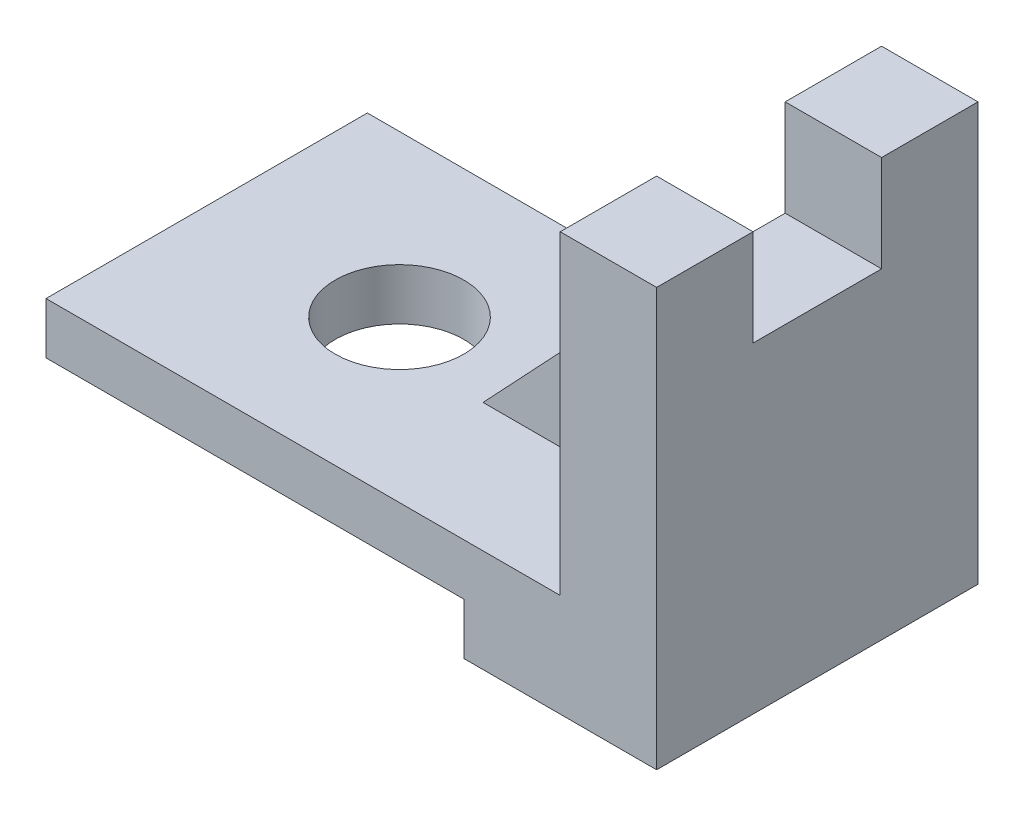
ISO-10303-21;
HEADER;
FILE_DESCRIPTION(('STEP AP214'),'2;1');
FILE_NAME('part.step','',(''),(''),'','','');
FILE_SCHEMA(('AUTOMOTIVE_DESIGN { 1 0 10303 214 1 1 1 1 }'));
ENDSEC;
DATA;
#1=APPLICATION_CONTEXT('core data for automotive mechanical design processes');
#2=APPLICATION_PROTOCOL_DEFINITION('international standard','automotive_design',2000,#1);
#3=PRODUCT_CONTEXT('',#1,'mechanical');
#4=PRODUCT('Part','Part','',(#3));
#5=PRODUCT_RELATED_PRODUCT_CATEGORY('part','',(#4));
#6=PRODUCT_DEFINITION_FORMATION('','',#4);
#7=PRODUCT_DEFINITION_CONTEXT('part definition',#1,'design');
#8=PRODUCT_DEFINITION('design','',#6,#7);
#9=PRODUCT_DEFINITION_SHAPE('','',#8);
#10=(LENGTH_UNIT() NAMED_UNIT(*) SI_UNIT(.MILLI.,.METRE.));
#11=(NAMED_UNIT(*) PLANE_ANGLE_UNIT() SI_UNIT($,.RADIAN.));
#12=(NAMED_UNIT(*) SI_UNIT($,.STERADIAN.) SOLID_ANGLE_UNIT());
#13=UNCERTAINTY_MEASURE_WITH_UNIT(LENGTH_MEASURE(1.E-05),#10,'distance_accuracy_value','');
#14=(GEOMETRIC_REPRESENTATION_CONTEXT(3) GLOBAL_UNCERTAINTY_ASSIGNED_CONTEXT((#13)) GLOBAL_UNIT_ASSIGNED_CONTEXT((#10,
#11,#12)) REPRESENTATION_CONTEXT('',''));
#15=CARTESIAN_POINT('',(0.,0.,0.));
#16=DIRECTION('',(0.,0.,1.));
#17=DIRECTION('',(1.,0.,0.));
#18=AXIS2_PLACEMENT_3D('',#15,#16,#17);
#19=CARTESIAN_POINT('',(-95.,16.,-25.));
#20=DIRECTION('',(0.,1.,0.));
#21=DIRECTION('',(0.,0.,1.));
#22=AXIS2_PLACEMENT_3D('',#19,#20,#21);
#23=PLANE('',#22);
#24=CARTESIAN_POINT('',(-65.,16.,0.));
#25=DIRECTION('',(0.,1.,0.));
#26=DIRECTION('',(0.,0.,1.));
#27=AXIS2_PLACEMENT_3D('',#24,#25,#26);
#28=CIRCLE('',#27,10.);
#29=CARTESIAN_POINT('',(-65.,16.,10.));
#30=VERTEX_POINT('',#29);
#31=EDGE_CURVE('E176',#30,#30,#28,.T.);
#32=ORIENTED_EDGE('',*,*,#31,.F.);
#33=EDGE_LOOP('',(#32));
#34=FACE_BOUND('',#33,.T.);
#35=DIRECTION('',(0.,0.,1.));
#36=VECTOR('',#35,1.);
#37=CARTESIAN_POINT('',(-15.,16.,-25.));
#38=LINE('',#37,#36);
#39=CARTESIAN_POINT('',(-15.,16.,5.));
#40=VERTEX_POINT('',#39);
#41=CARTESIAN_POINT('',(-15.,16.,25.));
#42=VERTEX_POINT('',#41);
#43=EDGE_CURVE('E167',#40,#42,#38,.T.);
#44=ORIENTED_EDGE('',*,*,#43,.F.);
#45=DIRECTION('',(1.,0.,0.));
#46=VECTOR('',#45,1.);
#47=CARTESIAN_POINT('',(-47.,16.,5.));
#48=LINE('',#47,#46);
#49=CARTESIAN_POINT('',(-47.,16.,5.));
#50=VERTEX_POINT('',#49);
#51=EDGE_CURVE('E147',#50,#40,#48,.T.);
#52=ORIENTED_EDGE('',*,*,#51,.F.);
#53=DIRECTION('',(0.,0.,-1.));
#54=VECTOR('',#53,1.);
#55=CARTESIAN_POINT('',(-47.,16.,5.));
#56=LINE('',#55,#54);
#57=CARTESIAN_POINT('',(-47.,16.,-5.));
#58=VERTEX_POINT('',#57);
#59=EDGE_CURVE('E156',#50,#58,#56,.T.);
#60=ORIENTED_EDGE('',*,*,#59,.T.);
#61=DIRECTION('',(1.,0.,0.));
#62=VECTOR('',#61,1.);
#63=CARTESIAN_POINT('',(-47.,16.,-5.));
#64=LINE('',#63,#62);
#65=CARTESIAN_POINT('',(-15.,16.,-5.));
#66=VERTEX_POINT('',#65);
#67=EDGE_CURVE('E173',#58,#66,#64,.T.);
#68=ORIENTED_EDGE('',*,*,#67,.T.);
#69=CARTESIAN_POINT('',(-15.,16.,-25.));
#70=VERTEX_POINT('',#69);
#71=EDGE_CURVE('E264',#70,#66,#38,.T.);
#72=ORIENTED_EDGE('',*,*,#71,.F.);
#73=DIRECTION('',(-1.,0.,0.));
#74=VECTOR('',#73,1.);
#75=CARTESIAN_POINT('',(-95.,16.,-25.));
#76=LINE('',#75,#74);
#77=CARTESIAN_POINT('',(-95.,16.,-25.));
#78=VERTEX_POINT('',#77);
#79=EDGE_CURVE('E242',#70,#78,#76,.T.);
#80=ORIENTED_EDGE('',*,*,#79,.T.);
#81=DIRECTION('',(0.,0.,1.));
#82=VECTOR('',#81,1.);
#83=CARTESIAN_POINT('',(-95.,16.,-25.));
#84=LINE('',#83,#82);
#85=CARTESIAN_POINT('',(-95.,16.,25.));
#86=VERTEX_POINT('',#85);
#87=EDGE_CURVE('E263',#78,#86,#84,.T.);
#88=ORIENTED_EDGE('',*,*,#87,.T.);
#89=DIRECTION('',(-1.,0.,0.));
#90=VECTOR('',#89,1.);
#91=CARTESIAN_POINT('',(-95.,16.,25.));
#92=LINE('',#91,#90);
#93=EDGE_CURVE('E217',#42,#86,#92,.T.);
#94=ORIENTED_EDGE('',*,*,#93,.F.);
#95=EDGE_LOOP('',(#44,#52,#60,#68,#72,#80,#88,#94));
#96=FACE_BOUND('',#95,.T.);
#97=ADVANCED_FACE('F41',(#34,#96),#23,.T.);
#98=CARTESIAN_POINT('',(-15.,16.,-25.));
#99=DIRECTION('',(-1.,0.,0.));
#100=DIRECTION('',(0.,0.,1.));
#101=AXIS2_PLACEMENT_3D('',#98,#99,#100);
#102=PLANE('',#101);
#103=DIRECTION('',(0.,0.,1.));
#104=VECTOR('',#103,1.);
#105=CARTESIAN_POINT('',(-15.,50.,-10.));
#106=LINE('',#105,#104);
#107=CARTESIAN_POINT('',(-15.,50.,5.));
#108=VERTEX_POINT('',#107);
#109=CARTESIAN_POINT('',(-15.,50.,10.));
#110=VERTEX_POINT('',#109);
#111=EDGE_CURVE('E192',#108,#110,#106,.T.);
#112=ORIENTED_EDGE('',*,*,#111,.F.);
#113=DIRECTION('',(0.,1.,0.));
#114=VECTOR('',#113,1.);
#115=CARTESIAN_POINT('',(-15.,16.,5.));
#116=LINE('',#115,#114);
#117=EDGE_CURVE('E59',#40,#108,#116,.T.);
#118=ORIENTED_EDGE('',*,*,#117,.F.);
#119=ORIENTED_EDGE('',*,*,#43,.T.);
#120=DIRECTION('',(0.,-1.,0.));
#121=VECTOR('',#120,1.);
#122=CARTESIAN_POINT('',(-15.,16.,25.));
#123=LINE('',#122,#121);
#124=CARTESIAN_POINT('',(-15.,65.,25.));
#125=VERTEX_POINT('',#124);
#126=EDGE_CURVE('E214',#125,#42,#123,.T.);
#127=ORIENTED_EDGE('',*,*,#126,.F.);
#128=DIRECTION('',(0.,0.,1.));
#129=VECTOR('',#128,1.);
#130=CARTESIAN_POINT('',(-15.,65.,-25.));
#131=LINE('',#130,#129);
#132=CARTESIAN_POINT('',(-15.,65.,10.));
#133=VERTEX_POINT('',#132);
#134=EDGE_CURVE('E267',#133,#125,#131,.T.);
#135=ORIENTED_EDGE('',*,*,#134,.F.);
#136=DIRECTION('',(0.,1.,0.));
#137=VECTOR('',#136,1.);
#138=CARTESIAN_POINT('',(-15.,50.,10.));
#139=LINE('',#138,#137);
#140=EDGE_CURVE('E186',#110,#133,#139,.T.);
#141=ORIENTED_EDGE('',*,*,#140,.F.);
#142=EDGE_LOOP('',(#112,#118,#119,#127,#135,#141));
#143=FACE_BOUND('',#142,.T.);
#144=ADVANCED_FACE('F310',(#143),#102,.T.);
#145=CARTESIAN_POINT('',(-15.,65.,-25.));
#146=DIRECTION('',(0.,1.,0.));
#147=DIRECTION('',(0.,0.,1.));
#148=AXIS2_PLACEMENT_3D('',#145,#146,#147);
#149=PLANE('',#148);
#150=DIRECTION('',(-1.,0.,0.));
#151=VECTOR('',#150,1.);
#152=CARTESIAN_POINT('',(0.,65.,10.));
#153=LINE('',#152,#151);
#154=CARTESIAN_POINT('',(0.,65.,10.));
#155=VERTEX_POINT('',#154);
#156=EDGE_CURVE('E199',#155,#133,#153,.T.);
#157=ORIENTED_EDGE('',*,*,#156,.T.);
#158=ORIENTED_EDGE('',*,*,#134,.T.);
#159=DIRECTION('',(-1.,0.,0.));
#160=VECTOR('',#159,1.);
#161=CARTESIAN_POINT('',(-15.,65.,25.));
#162=LINE('',#161,#160);
#163=CARTESIAN_POINT('',(0.,65.,25.));
#164=VERTEX_POINT('',#163);
#165=EDGE_CURVE('E215',#164,#125,#162,.T.);
#166=ORIENTED_EDGE('',*,*,#165,.F.);
#167=DIRECTION('',(0.,0.,1.));
#168=VECTOR('',#167,1.);
#169=CARTESIAN_POINT('',(0.,65.,-25.));
#170=LINE('',#169,#168);
#171=EDGE_CURVE('E258',#155,#164,#170,.T.);
#172=ORIENTED_EDGE('',*,*,#171,.F.);
#173=EDGE_LOOP('',(#157,#158,#166,#172));
#174=FACE_BOUND('',#173,.T.);
#175=ADVANCED_FACE('F276',(#174),#149,.T.);
#176=CARTESIAN_POINT('',(0.,65.,-25.));
#177=DIRECTION('',(1.,0.,0.));
#178=DIRECTION('',(0.,1.,0.));
#179=AXIS2_PLACEMENT_3D('',#176,#177,#178);
#180=PLANE('',#179);
#181=DIRECTION('',(0.,1.,0.));
#182=VECTOR('',#181,1.);
#183=CARTESIAN_POINT('',(0.,50.,10.));
#184=LINE('',#183,#182);
#185=CARTESIAN_POINT('',(0.,50.,10.));
#186=VERTEX_POINT('',#185);
#187=EDGE_CURVE('E188',#186,#155,#184,.T.);
#188=ORIENTED_EDGE('',*,*,#187,.T.);
#189=ORIENTED_EDGE('',*,*,#171,.T.);
#190=DIRECTION('',(0.,1.,0.));
#191=VECTOR('',#190,1.);
#192=CARTESIAN_POINT('',(0.,65.,25.));
#193=LINE('',#192,#191);
#194=CARTESIAN_POINT('',(0.,0.,25.));
#195=VERTEX_POINT('',#194);
#196=EDGE_CURVE('E201',#195,#164,#193,.T.);
#197=ORIENTED_EDGE('',*,*,#196,.F.);
#198=DIRECTION('',(0.,0.,1.));
#199=VECTOR('',#198,1.);
#200=CARTESIAN_POINT('',(0.,0.,-25.));
#201=LINE('',#200,#199);
#202=CARTESIAN_POINT('',(0.,0.,-25.));
#203=VERTEX_POINT('',#202);
#204=EDGE_CURVE('E11',#203,#195,#201,.T.);
#205=ORIENTED_EDGE('',*,*,#204,.F.);
#206=DIRECTION('',(0.,1.,0.));
#207=VECTOR('',#206,1.);
#208=CARTESIAN_POINT('',(0.,65.,-25.));
#209=LINE('',#208,#207);
#210=CARTESIAN_POINT('',(0.,65.,-25.));
#211=VERTEX_POINT('',#210);
#212=EDGE_CURVE('E235',#203,#211,#209,.T.);
#213=ORIENTED_EDGE('',*,*,#212,.T.);
#214=CARTESIAN_POINT('',(0.,65.,-10.));
#215=VERTEX_POINT('',#214);
#216=EDGE_CURVE('E44',#211,#215,#170,.T.);
#217=ORIENTED_EDGE('',*,*,#216,.T.);
#218=DIRECTION('',(0.,-1.,0.));
#219=VECTOR('',#218,1.);
#220=CARTESIAN_POINT('',(0.,65.,-10.));
#221=LINE('',#220,#219);
#222=CARTESIAN_POINT('',(0.,50.,-10.));
#223=VERTEX_POINT('',#222);
#224=EDGE_CURVE('E69',#215,#223,#221,.T.);
#225=ORIENTED_EDGE('',*,*,#224,.T.);
#226=DIRECTION('',(0.,0.,1.));
#227=VECTOR('',#226,1.);
#228=CARTESIAN_POINT('',(0.,50.,-10.));
#229=LINE('',#228,#227);
#230=EDGE_CURVE('E183',#223,#186,#229,.T.);
#231=ORIENTED_EDGE('',*,*,#230,.T.);
#232=EDGE_LOOP('',(#188,#189,#197,#205,#213,#217,#225,#231));
#233=FACE_BOUND('',#232,.T.);
#234=ADVANCED_FACE('F43',(#233),#180,.T.);
#235=CARTESIAN_POINT('',(0.,0.,-25.));
#236=DIRECTION('',(0.,-1.,0.));
#237=DIRECTION('',(0.,0.,-1.));
#238=AXIS2_PLACEMENT_3D('',#235,#236,#237);
#239=PLANE('',#238);
#240=ORIENTED_EDGE('',*,*,#204,.T.);
#241=DIRECTION('',(1.,0.,0.));
#242=VECTOR('',#241,1.);
#243=CARTESIAN_POINT('',(0.,0.,25.));
#244=LINE('',#243,#242);
#245=CARTESIAN_POINT('',(-30.,0.,25.));
#246=VERTEX_POINT('',#245);
#247=EDGE_CURVE('E230',#246,#195,#244,.T.);
#248=ORIENTED_EDGE('',*,*,#247,.F.);
#249=DIRECTION('',(0.,0.,1.));
#250=VECTOR('',#249,1.);
#251=CARTESIAN_POINT('',(-30.,0.,-25.));
#252=LINE('',#251,#250);
#253=CARTESIAN_POINT('',(-30.,0.,-25.));
#254=VERTEX_POINT('',#253);
#255=EDGE_CURVE('E49',#254,#246,#252,.T.);
#256=ORIENTED_EDGE('',*,*,#255,.F.);
#257=DIRECTION('',(1.,0.,0.));
#258=VECTOR('',#257,1.);
#259=CARTESIAN_POINT('',(0.,0.,-25.));
#260=LINE('',#259,#258);
#261=EDGE_CURVE('E255',#254,#203,#260,.T.);
#262=ORIENTED_EDGE('',*,*,#261,.T.);
#263=EDGE_LOOP('',(#240,#248,#256,#262));
#264=FACE_BOUND('',#263,.T.);
#265=ADVANCED_FACE('F289',(#264),#239,.T.);
#266=CARTESIAN_POINT('',(-30.,0.,-25.));
#267=DIRECTION('',(-1.,0.,0.));
#268=DIRECTION('',(0.,0.,1.));
#269=AXIS2_PLACEMENT_3D('',#266,#267,#268);
#270=PLANE('',#269);
#271=ORIENTED_EDGE('',*,*,#255,.T.);
#272=DIRECTION('',(0.,-1.,0.));
#273=VECTOR('',#272,1.);
#274=CARTESIAN_POINT('',(-30.,0.,25.));
#275=LINE('',#274,#273);
#276=CARTESIAN_POINT('',(-30.,8.,25.));
#277=VERTEX_POINT('',#276);
#278=EDGE_CURVE('E227',#277,#246,#275,.T.);
#279=ORIENTED_EDGE('',*,*,#278,.F.);
#280=DIRECTION('',(0.,0.,1.));
#281=VECTOR('',#280,1.);
#282=CARTESIAN_POINT('',(-30.,8.,-25.));
#283=LINE('',#282,#281);
#284=CARTESIAN_POINT('',(-30.,8.,-25.));
#285=VERTEX_POINT('',#284);
#286=EDGE_CURVE('E259',#285,#277,#283,.T.);
#287=ORIENTED_EDGE('',*,*,#286,.F.);
#288=DIRECTION('',(0.,-1.,0.));
#289=VECTOR('',#288,1.);
#290=CARTESIAN_POINT('',(-30.,0.,-25.));
#291=LINE('',#290,#289);
#292=EDGE_CURVE('E253',#285,#254,#291,.T.);
#293=ORIENTED_EDGE('',*,*,#292,.T.);
#294=EDGE_LOOP('',(#271,#279,#287,#293));
#295=FACE_BOUND('',#294,.T.);
#296=ADVANCED_FACE('F317',(#295),#270,.T.);
#297=CARTESIAN_POINT('',(-30.,8.,-25.));
#298=DIRECTION('',(0.,-1.,0.));
#299=DIRECTION('',(1.,0.,0.));
#300=AXIS2_PLACEMENT_3D('',#297,#298,#299);
#301=PLANE('',#300);
#302=CARTESIAN_POINT('',(-65.,7.99999999999999,0.));
#303=DIRECTION('',(0.,1.,0.));
#304=DIRECTION('',(0.,0.,1.));
#305=AXIS2_PLACEMENT_3D('',#302,#303,#304);
#306=CIRCLE('',#305,10.);
#307=CARTESIAN_POINT('',(-65.,7.99999999999999,10.));
#308=VERTEX_POINT('',#307);
#309=EDGE_CURVE('E180',#308,#308,#306,.T.);
#310=ORIENTED_EDGE('',*,*,#309,.T.);
#311=EDGE_LOOP('',(#310));
#312=FACE_BOUND('',#311,.T.);
#313=ORIENTED_EDGE('',*,*,#286,.T.);
#314=DIRECTION('',(1.,0.,0.));
#315=VECTOR('',#314,1.);
#316=CARTESIAN_POINT('',(-30.,8.,25.));
#317=LINE('',#316,#315);
#318=CARTESIAN_POINT('',(-95.,7.99999999999999,25.));
#319=VERTEX_POINT('',#318);
#320=EDGE_CURVE('E221',#319,#277,#317,.T.);
#321=ORIENTED_EDGE('',*,*,#320,.F.);
#322=DIRECTION('',(0.,0.,1.));
#323=VECTOR('',#322,1.);
#324=CARTESIAN_POINT('',(-95.,7.99999999999999,-25.));
#325=LINE('',#324,#323);
#326=CARTESIAN_POINT('',(-95.,7.99999999999999,-25.));
#327=VERTEX_POINT('',#326);
#328=EDGE_CURVE('E261',#327,#319,#325,.T.);
#329=ORIENTED_EDGE('',*,*,#328,.F.);
#330=DIRECTION('',(1.,0.,0.));
#331=VECTOR('',#330,1.);
#332=CARTESIAN_POINT('',(-30.,8.,-25.));
#333=LINE('',#332,#331);
#334=EDGE_CURVE('E250',#327,#285,#333,.T.);
#335=ORIENTED_EDGE('',*,*,#334,.T.);
#336=EDGE_LOOP('',(#313,#321,#329,#335));
#337=FACE_BOUND('',#336,.T.);
#338=ADVANCED_FACE('F316',(#312,#337),#301,.T.);
#339=CARTESIAN_POINT('',(-95.,7.99999999999999,-25.));
#340=DIRECTION('',(-1.,0.,0.));
#341=DIRECTION('',(0.,0.,1.));
#342=AXIS2_PLACEMENT_3D('',#339,#340,#341);
#343=PLANE('',#342);
#344=ORIENTED_EDGE('',*,*,#328,.T.);
#345=DIRECTION('',(0.,-1.,0.));
#346=VECTOR('',#345,1.);
#347=CARTESIAN_POINT('',(-95.,7.99999999999999,25.));
#348=LINE('',#347,#346);
#349=EDGE_CURVE('E222',#86,#319,#348,.T.);
#350=ORIENTED_EDGE('',*,*,#349,.F.);
#351=ORIENTED_EDGE('',*,*,#87,.F.);
#352=DIRECTION('',(0.,-1.,0.));
#353=VECTOR('',#352,1.);
#354=CARTESIAN_POINT('',(-95.,7.99999999999999,-25.));
#355=LINE('',#354,#353);
#356=EDGE_CURVE('E245',#78,#327,#355,.T.);
#357=ORIENTED_EDGE('',*,*,#356,.T.);
#358=EDGE_LOOP('',(#344,#350,#351,#357));
#359=FACE_BOUND('',#358,.T.);
#360=ADVANCED_FACE('F311',(#359),#343,.T.);
#361=DIRECTION('',(0.,1.,0.));
#362=VECTOR('',#361,1.);
#363=CARTESIAN_POINT('',(-15.,16.,-5.));
#364=LINE('',#363,#362);
#365=CARTESIAN_POINT('',(-15.,50.,-5.));
#366=VERTEX_POINT('',#365);
#367=EDGE_CURVE('E168',#66,#366,#364,.T.);
#368=ORIENTED_EDGE('',*,*,#367,.T.);
#369=CARTESIAN_POINT('',(-15.,50.,-10.));
#370=VERTEX_POINT('',#369);
#371=EDGE_CURVE('E198',#370,#366,#106,.T.);
#372=ORIENTED_EDGE('',*,*,#371,.F.);
#373=DIRECTION('',(0.,-1.,0.));
#374=VECTOR('',#373,1.);
#375=CARTESIAN_POINT('',(-15.,65.,-10.));
#376=LINE('',#375,#374);
#377=CARTESIAN_POINT('',(-15.,65.,-10.));
#378=VERTEX_POINT('',#377);
#379=EDGE_CURVE('E182',#378,#370,#376,.T.);
#380=ORIENTED_EDGE('',*,*,#379,.F.);
#381=CARTESIAN_POINT('',(-15.,65.,-25.));
#382=VERTEX_POINT('',#381);
#383=EDGE_CURVE('E270',#382,#378,#131,.T.);
#384=ORIENTED_EDGE('',*,*,#383,.F.);
#385=DIRECTION('',(0.,-1.,0.));
#386=VECTOR('',#385,1.);
#387=CARTESIAN_POINT('',(-15.,16.,-25.));
#388=LINE('',#387,#386);
#389=EDGE_CURVE('E239',#382,#70,#388,.T.);
#390=ORIENTED_EDGE('',*,*,#389,.T.);
#391=ORIENTED_EDGE('',*,*,#71,.T.);
#392=EDGE_LOOP('',(#368,#372,#380,#384,#390,#391));
#393=FACE_BOUND('',#392,.T.);
#394=ADVANCED_FACE('F300',(#393),#102,.T.);
#395=DIRECTION('',(-1.,0.,0.));
#396=VECTOR('',#395,1.);
#397=CARTESIAN_POINT('',(0.,65.,-10.));
#398=LINE('',#397,#396);
#399=EDGE_CURVE('E191',#215,#378,#398,.T.);
#400=ORIENTED_EDGE('',*,*,#399,.F.);
#401=ORIENTED_EDGE('',*,*,#216,.F.);
#402=DIRECTION('',(-1.,0.,0.));
#403=VECTOR('',#402,1.);
#404=CARTESIAN_POINT('',(-15.,65.,-25.));
#405=LINE('',#404,#403);
#406=EDGE_CURVE('E237',#211,#382,#405,.T.);
#407=ORIENTED_EDGE('',*,*,#406,.T.);
#408=ORIENTED_EDGE('',*,*,#383,.T.);
#409=EDGE_LOOP('',(#400,#401,#407,#408));
#410=FACE_BOUND('',#409,.T.);
#411=ADVANCED_FACE('F293',(#410),#149,.T.);
#412=CARTESIAN_POINT('',(0.,0.,-25.));
#413=DIRECTION('',(0.,0.,-1.));
#414=DIRECTION('',(-1.,0.,0.));
#415=AXIS2_PLACEMENT_3D('',#412,#413,#414);
#416=PLANE('',#415);
#417=ORIENTED_EDGE('',*,*,#212,.F.);
#418=ORIENTED_EDGE('',*,*,#261,.F.);
#419=ORIENTED_EDGE('',*,*,#292,.F.);
#420=ORIENTED_EDGE('',*,*,#334,.F.);
#421=ORIENTED_EDGE('',*,*,#356,.F.);
#422=ORIENTED_EDGE('',*,*,#79,.F.);
#423=ORIENTED_EDGE('',*,*,#389,.F.);
#424=ORIENTED_EDGE('',*,*,#406,.F.);
#425=EDGE_LOOP('',(#417,#418,#419,#420,#421,#422,#423,#424));
#426=FACE_BOUND('',#425,.T.);
#427=ADVANCED_FACE('F292',(#426),#416,.T.);
#428=CARTESIAN_POINT('',(0.,0.,25.));
#429=DIRECTION('',(0.,0.,-1.));
#430=DIRECTION('',(-1.,0.,0.));
#431=AXIS2_PLACEMENT_3D('',#428,#429,#430);
#432=PLANE('',#431);
#433=ORIENTED_EDGE('',*,*,#196,.T.);
#434=ORIENTED_EDGE('',*,*,#165,.T.);
#435=ORIENTED_EDGE('',*,*,#126,.T.);
#436=ORIENTED_EDGE('',*,*,#93,.T.);
#437=ORIENTED_EDGE('',*,*,#349,.T.);
#438=ORIENTED_EDGE('',*,*,#320,.T.);
#439=ORIENTED_EDGE('',*,*,#278,.T.);
#440=ORIENTED_EDGE('',*,*,#247,.T.);
#441=EDGE_LOOP('',(#433,#434,#435,#436,#437,#438,#439,#440));
#442=FACE_BOUND('',#441,.T.);
#443=ADVANCED_FACE('F282',(#442),#432,.F.);
#444=CARTESIAN_POINT('',(0.,50.,10.));
#445=DIRECTION('',(0.,0.,1.));
#446=DIRECTION('',(1.,0.,0.));
#447=AXIS2_PLACEMENT_3D('',#444,#445,#446);
#448=PLANE('',#447);
#449=ORIENTED_EDGE('',*,*,#140,.T.);
#450=ORIENTED_EDGE('',*,*,#156,.F.);
#451=ORIENTED_EDGE('',*,*,#187,.F.);
#452=DIRECTION('',(-1.,0.,0.));
#453=VECTOR('',#452,1.);
#454=CARTESIAN_POINT('',(0.,50.,10.));
#455=LINE('',#454,#453);
#456=EDGE_CURVE('E204',#186,#110,#455,.T.);
#457=ORIENTED_EDGE('',*,*,#456,.T.);
#458=EDGE_LOOP('',(#449,#450,#451,#457));
#459=FACE_BOUND('',#458,.T.);
#460=ADVANCED_FACE('F307',(#459),#448,.F.);
#461=CARTESIAN_POINT('',(0.,50.,-10.));
#462=DIRECTION('',(0.,-1.,0.));
#463=DIRECTION('',(0.,0.,-1.));
#464=AXIS2_PLACEMENT_3D('',#461,#462,#463);
#465=PLANE('',#464);
#466=ORIENTED_EDGE('',*,*,#371,.T.);
#467=DIRECTION('',(0.,0.,-1.));
#468=VECTOR('',#467,1.);
#469=CARTESIAN_POINT('',(-15.,50.,5.));
#470=LINE('',#469,#468);
#471=EDGE_CURVE('E165',#108,#366,#470,.T.);
#472=ORIENTED_EDGE('',*,*,#471,.F.);
#473=ORIENTED_EDGE('',*,*,#111,.T.);
#474=ORIENTED_EDGE('',*,*,#456,.F.);
#475=ORIENTED_EDGE('',*,*,#230,.F.);
#476=DIRECTION('',(-1.,0.,0.));
#477=VECTOR('',#476,1.);
#478=CARTESIAN_POINT('',(0.,50.,-10.));
#479=LINE('',#478,#477);
#480=EDGE_CURVE('E210',#223,#370,#479,.T.);
#481=ORIENTED_EDGE('',*,*,#480,.T.);
#482=EDGE_LOOP('',(#466,#472,#473,#474,#475,#481));
#483=FACE_BOUND('',#482,.T.);
#484=ADVANCED_FACE('F305',(#483),#465,.F.);
#485=CARTESIAN_POINT('',(0.,65.,-10.));
#486=DIRECTION('',(0.,0.,-1.));
#487=DIRECTION('',(0.,1.,0.));
#488=AXIS2_PLACEMENT_3D('',#485,#486,#487);
#489=PLANE('',#488);
#490=ORIENTED_EDGE('',*,*,#379,.T.);
#491=ORIENTED_EDGE('',*,*,#480,.F.);
#492=ORIENTED_EDGE('',*,*,#224,.F.);
#493=ORIENTED_EDGE('',*,*,#399,.T.);
#494=EDGE_LOOP('',(#490,#491,#492,#493));
#495=FACE_BOUND('',#494,.T.);
#496=ADVANCED_FACE('F297',(#495),#489,.F.);
#497=CARTESIAN_POINT('',(-65.,7.99999999999999,0.));
#498=DIRECTION('',(0.,1.,0.));
#499=DIRECTION('',(0.,0.,1.));
#500=AXIS2_PLACEMENT_3D('',#497,#498,#499);
#501=CYLINDRICAL_SURFACE('',#500,10.);
#502=ORIENTED_EDGE('',*,*,#309,.F.);
#503=EDGE_LOOP('',(#502));
#504=FACE_BOUND('',#503,.T.);
#505=ORIENTED_EDGE('',*,*,#31,.T.);
#506=EDGE_LOOP('',(#505));
#507=FACE_BOUND('',#506,.T.);
#508=ADVANCED_FACE('F427',(#504,#507),#501,.F.);
#509=CARTESIAN_POINT('',(-15.,50.,5.));
#510=DIRECTION('',(0.728199992692803,-0.685364699004991,0.));
#511=DIRECTION('',(0.685364699004991,0.728199992692803,0.));
#512=AXIS2_PLACEMENT_3D('',#509,#510,#511);
#513=PLANE('',#512);
#514=DIRECTION('',(-0.685364699004991,-0.728199992692803,0.));
#515=VECTOR('',#514,1.);
#516=CARTESIAN_POINT('',(-15.,50.,-5.));
#517=LINE('',#516,#515);
#518=EDGE_CURVE('E158',#366,#58,#517,.T.);
#519=ORIENTED_EDGE('',*,*,#518,.T.);
#520=ORIENTED_EDGE('',*,*,#59,.F.);
#521=DIRECTION('',(-0.685364699004991,-0.728199992692803,0.));
#522=VECTOR('',#521,1.);
#523=CARTESIAN_POINT('',(-15.,50.,5.));
#524=LINE('',#523,#522);
#525=EDGE_CURVE('E148',#108,#50,#524,.T.);
#526=ORIENTED_EDGE('',*,*,#525,.F.);
#527=ORIENTED_EDGE('',*,*,#471,.T.);
#528=EDGE_LOOP('',(#519,#520,#526,#527));
#529=FACE_BOUND('',#528,.T.);
#530=ADVANCED_FACE('F160',(#529),#513,.F.);
#531=CARTESIAN_POINT('',(0.,0.,5.));
#532=DIRECTION('',(0.,0.,-1.));
#533=DIRECTION('',(-1.,0.,0.));
#534=AXIS2_PLACEMENT_3D('',#531,#532,#533);
#535=PLANE('',#534);
#536=ORIENTED_EDGE('',*,*,#117,.T.);
#537=ORIENTED_EDGE('',*,*,#525,.T.);
#538=ORIENTED_EDGE('',*,*,#51,.T.);
#539=EDGE_LOOP('',(#536,#537,#538));
#540=FACE_BOUND('',#539,.T.);
#541=ADVANCED_FACE('F146',(#540),#535,.F.);
#542=CARTESIAN_POINT('',(0.,0.,-5.));
#543=DIRECTION('',(0.,0.,-1.));
#544=DIRECTION('',(-1.,0.,0.));
#545=AXIS2_PLACEMENT_3D('',#542,#543,#544);
#546=PLANE('',#545);
#547=ORIENTED_EDGE('',*,*,#367,.F.);
#548=ORIENTED_EDGE('',*,*,#67,.F.);
#549=ORIENTED_EDGE('',*,*,#518,.F.);
#550=EDGE_LOOP('',(#547,#548,#549));
#551=FACE_BOUND('',#550,.T.);
#552=ADVANCED_FACE('F464',(#551),#546,.T.);
#553=CLOSED_SHELL('',(#97,#144,#175,#234,#265,#296,#338,#360,#394,#411,#427,#443,#460,#484,#496,
#508,#530,#541,#552));
#554=MANIFOLD_SOLID_BREP('B2',#553);
#555=ADVANCED_BREP_SHAPE_REPRESENTATION('',(#18,#554),#14);
#556=SHAPE_DEFINITION_REPRESENTATION(#9,#555);
ENDSEC;
END-ISO-10303-21;
